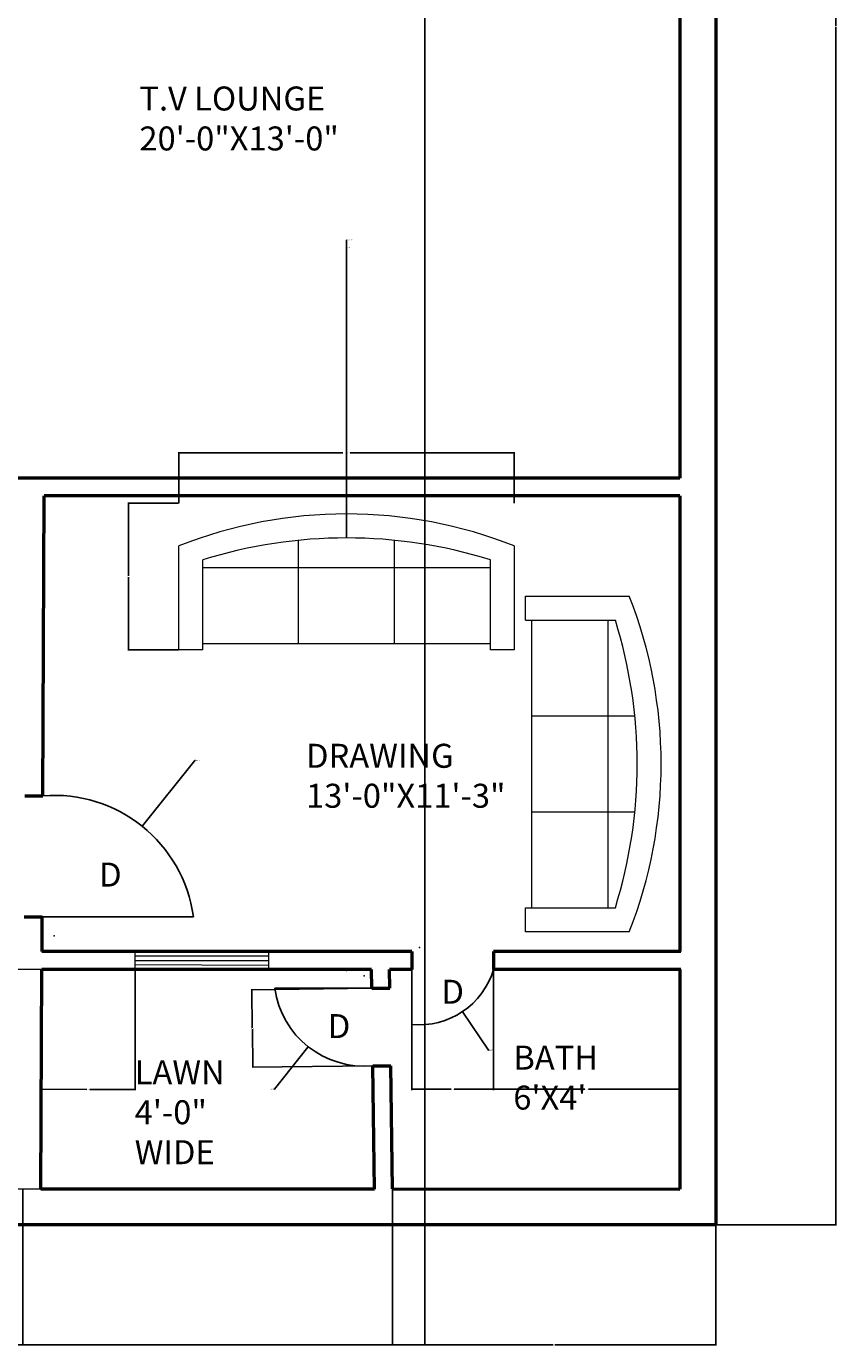
# Model space of a CAD drawing. Units: inches. Extents: x 2341 to 2761, y 2129 to 2789.
# Tile 2 of 4: x 2559 to 2761, y 2129 to 2459. Entities that reach past the tile are written whole.
import ezdxf

# ---------------------------------------------------------------- set-up
doc = ezdxf.new("R2010")
doc.units = ezdxf.units.IN
for name, color, linetype, lineweight in [('A-ANNO-DIMS', 2, 'Continuous', 18), ('A-ANNO-TEXT', 7, 'Continuous', 18), ('A-AREA-IDEN', 7, 'Continuous', 25), ('A-DOOR', 3, 'Continuous', 25), ('A-FURN', 8, 'Continuous', 18), ('A-GLAZ', 4, 'Continuous', 18), ('A-WALL', 7, 'Continuous', 50)]:
    doc.layers.add(name, color=color, linetype=linetype, lineweight=lineweight)
doc.styles.get("Standard").update_dxf_attribs({"font": 'arial.ttf'})
doc.dimstyles.get("Standard").update_dxf_attribs({"dimtxt": 0.18, "dimasz": 0.18, "dimexe": 0.18, "dimexo": 0.0625, "dimgap": 0.09, "dimtad": 0, "dimtih": 1, "dimtoh": 1, "dimdec": 4, "dimzin": 0, "dimdsep": 46, "dimtxsty": 'Standard', "dimcen": 0.09, "dimadec": 0, "dimazin": 0, "dimtfac": 1, "dimtdec": 4, "dimtofl": 0, "dimtmove": 0, "dimatfit": 3, "dimfxl": 1, "dimtolj": 1, "dimtzin": 0, "dimarcsym": 0})

# ---------------------------------------------------------------- blocks, each defined once
blk = doc.blocks.new('Sofa - Roundback 7 ft.')
for p, q in [((-12.00002, -32.4421), (-12.00003, -6.5971)), ((11.99997, -32.4421), (11.99998, -6.5971)), ((-36.000027, -34), (-36.000027, -11.4696)), ((35.99998, -34), (35.99998, -11.4696)), ((-35.999844, -13.3819), (35.9998, -13.3819)), ((-36.000027, -32.4421), (35.99998, -32.4421))]:
    blk.add_line(p, q)
for points in [[(-36.000027, -34), (-42.000027, -34), (-42.000027, -8)], [(41.99998, -8), (41.99998, -34), (35.99998, -34)]]:
    blk.add_lwpolyline(points)
for centre, radius, start, end in [((0, -114.25), 114.25, 68.43141, 111.5686), ((-0.00001, -127.1968), 121.1968, 72.72033, 107.2797)]:
    blk.add_arc(centre, radius, start, end)
blk = doc.blocks.new('WIN-33IN-NARROW')
for p, q in [((0, 3.43), (33.34, 3.43)), ((0, 2.27), (33.34, 2.27)), ((0, 1.23), (33.34, 1.12))]:
    blk.add_line(p, q)
blk.add_lwpolyline([(0, 4.54), (33.34, 4.54), (33.34, 0), (0, 0)], close=True)
blk = doc.blocks.new('*D9')
at = {"layer": 'A-ANNO-DIMS', "color": 0, "lineweight": -2, "transparency": 16777216}
for p, q in [((2596.77, 2339.82), (2596.77, 2352.54)), ((2596.95, 2352.36), (2637.86, 2352.36)), ((2680.59, 2352.36), (2639.67, 2352.36)), ((2680.77, 2339.82), (2680.77, 2352.54))]:
    blk.add_line(p, q, dxfattribs=at)
at = {"layer": 'A-ANNO-DIMS', "color": 0, "transparency": 16777216}
for points in [[(2596.95, 2352.39), (2596.95, 2352.33), (2596.77, 2352.36)], [(2680.59, 2352.39), (2680.59, 2352.33), (2680.77, 2352.36)]]:
    blk.add_solid(points, dxfattribs=at)
at = {"layer": 'Defpoints', "color": 0, "transparency": 16777216}
for p in [(2680.77, 2352.36), (2596.77, 2339.76), (2680.77, 2339.76)]:
    blk.add_point(p, dxfattribs=at)
at = {"layer": 'A-ANNO-DIMS', "color": 0, "transparency": 16777216, "insert": (2638.77, 2352.36), "char_height": 0.18, "attachment_point": 5}
blk.add_mtext('\\A1;SOFA 84 TYP.', dxfattribs=at)
blk = doc.blocks.new('*D10')
at = {"layer": 'A-ANNO-DIMS', "color": 0, "lineweight": -2, "transparency": 16777216}
for p, q in [((2596.71, 2339.76), (2583.99, 2339.76)), ((2584.17, 2339.58), (2584.17, 2321.61)), ((2584.17, 2303.27), (2584.17, 2321.24)), ((2596.71, 2303.09), (2583.99, 2303.09))]:
    blk.add_line(p, q, dxfattribs=at)
at = {"layer": 'A-ANNO-DIMS', "color": 0, "transparency": 16777216}
for points in [[(2584.14, 2339.58), (2584.2, 2339.58), (2584.17, 2339.76)], [(2584.14, 2303.27), (2584.2, 2303.27), (2584.17, 2303.09)]]:
    blk.add_solid(points, dxfattribs=at)
at = {"layer": 'Defpoints', "color": 0, "transparency": 16777216}
for p in [(2584.17, 2339.76), (2596.77, 2339.76), (2596.77, 2303.09)]:
    blk.add_point(p, dxfattribs=at)
at = {"layer": 'A-ANNO-DIMS', "color": 0, "transparency": 16777216, "insert": (2584.17, 2321.42), "char_height": 0.18, "attachment_point": 5}
blk.add_mtext('\\A1;37 TYP.', dxfattribs=at)
blk = doc.blocks.new('*D12')
at = {"layer": 'A-ANNO-DIMS', "color": 0, "lineweight": -2, "transparency": 16777216}
for p, q in [((2731.3, 2759.12), (2761.44, 2759.12)), ((2761.26, 2758.94), (2761.26, 2459.3)), ((2761.26, 2159.3), (2761.26, 2458.94)), ((2731.3, 2159.12), (2761.44, 2159.12))]:
    blk.add_line(p, q, dxfattribs=at)
at = {"layer": 'A-ANNO-DIMS', "color": 0, "transparency": 16777216}
for points in [[(2761.23, 2758.94), (2761.29, 2758.94), (2761.26, 2759.12)], [(2761.23, 2159.3), (2761.29, 2159.3), (2761.26, 2159.12)]]:
    blk.add_solid(points, dxfattribs=at)
at = {"layer": 'Defpoints', "color": 0, "transparency": 16777216}
for p in [(2731.24, 2759.12), (2761.26, 2759.12), (2731.24, 2159.12)]:
    blk.add_point(p, dxfattribs=at)
at = {"layer": 'A-ANNO-DIMS', "color": 0, "transparency": 16777216, "insert": (2761.26, 2459.12), "char_height": 0.18, "attachment_point": 5}
blk.add_mtext('\\A1;600', dxfattribs=at)
blk = doc.blocks.new('*D17')
at = {"layer": 'A-ANNO-DIMS', "color": 0, "lineweight": -2, "transparency": 16777216}
for p, q in [((2444.74, 2750.05), (2444.74, 2128.92)), ((2658.39, 2749.97), (2658.39, 2128.92)), ((2444.92, 2129.1), (2551.1, 2129.1)), ((2658.21, 2129.1), (2552.03, 2129.1))]:
    blk.add_line(p, q, dxfattribs=at)
at = {"layer": 'A-ANNO-DIMS', "color": 0, "transparency": 16777216}
for points in [[(2444.92, 2129.13), (2444.92, 2129.07), (2444.74, 2129.1)], [(2658.21, 2129.13), (2658.21, 2129.07), (2658.39, 2129.1)]]:
    blk.add_solid(points, dxfattribs=at)
at = {"layer": 'Defpoints', "color": 0, "transparency": 16777216}
for p in [(2444.74, 2750.12), (2658.39, 2750.04), (2658.39, 2129.1)]:
    blk.add_point(p, dxfattribs=at)
at = {"layer": 'A-ANNO-DIMS', "color": 0, "transparency": 16777216, "insert": (2551.56, 2129.1), "char_height": 0.18, "attachment_point": 5}
blk.add_mtext('\\A1;213.65', dxfattribs=at)
blk = doc.blocks.new('*D25')
at = {"layer": 'A-ANNO-DIMS', "color": 0, "lineweight": -2, "transparency": 16777216}
for p, q in [((2557.74, 2168.07), (2557.74, 2128.92)), ((2650.24, 2168.1), (2650.24, 2128.92)), ((2557.92, 2129.1), (2603.67, 2129.1)), ((2650.06, 2129.1), (2604.32, 2129.1))]:
    blk.add_line(p, q, dxfattribs=at)
at = {"layer": 'A-ANNO-DIMS', "color": 0, "transparency": 16777216}
for points in [[(2557.92, 2129.13), (2557.92, 2129.07), (2557.74, 2129.1)], [(2650.06, 2129.13), (2650.06, 2129.07), (2650.24, 2129.1)]]:
    blk.add_solid(points, dxfattribs=at)
at = {"layer": 'Defpoints', "color": 0, "transparency": 16777216}
for p in [(2557.74, 2168.13), (2650.24, 2168.16), (2650.24, 2129.1)]:
    blk.add_point(p, dxfattribs=at)
at = {"layer": 'A-ANNO-DIMS', "color": 0, "transparency": 16777216, "insert": (2603.99, 2129.1), "char_height": 0.18, "attachment_point": 5}
blk.add_mtext('\\A1;92.5', dxfattribs=at)
blk = doc.blocks.new('*D26')
at = {"layer": 'A-ANNO-DIMS', "color": 0, "lineweight": -2, "transparency": 16777216}
for p, q in [((2650.24, 2168.1), (2650.24, 2128.92)), ((2731.24, 2159.06), (2731.24, 2128.92)), ((2650.42, 2129.1), (2690.54, 2129.1)), ((2731.06, 2129.1), (2690.94, 2129.1))]:
    blk.add_line(p, q, dxfattribs=at)
at = {"layer": 'A-ANNO-DIMS', "color": 0, "transparency": 16777216}
for points in [[(2650.42, 2129.13), (2650.42, 2129.07), (2650.24, 2129.1)], [(2731.06, 2129.13), (2731.06, 2129.07), (2731.24, 2129.1)]]:
    blk.add_solid(points, dxfattribs=at)
at = {"layer": 'Defpoints', "color": 0, "transparency": 16777216}
for p in [(2650.24, 2168.16), (2731.24, 2159.12), (2731.24, 2129.1)]:
    blk.add_point(p, dxfattribs=at)
at = {"layer": 'A-ANNO-DIMS', "color": 0, "transparency": 16777216, "insert": (2690.74, 2129.1), "char_height": 0.18, "attachment_point": 5}
blk.add_mtext('\\A1;81', dxfattribs=at)
blk = doc.blocks.new('*D30')
at = {"layer": 'A-ANNO-DIMS', "color": 0, "lineweight": -2, "transparency": 16777216}
for p, q in [((2562.45, 2223.1), (2532.31, 2223.25)), ((2532.49, 2223.06), (2532.36, 2195.94)), ((2532.22, 2168.45), (2532.36, 2195.58)), ((2562.18, 2168.12), (2532.04, 2168.27))]:
    blk.add_line(p, q, dxfattribs=at)
at = {"layer": 'A-ANNO-DIMS', "color": 0, "transparency": 16777216}
for points in [[(2532.46, 2223.06), (2532.52, 2223.06), (2532.49, 2223.24)], [(2532.19, 2168.45), (2532.25, 2168.45), (2532.22, 2168.27)]]:
    blk.add_solid(points, dxfattribs=at)
at = {"layer": 'Defpoints', "color": 0, "transparency": 16777216}
for p in [(2532.49, 2223.24), (2562.51, 2223.1), (2562.24, 2168.12)]:
    blk.add_point(p, dxfattribs=at)
at = {"layer": 'A-ANNO-DIMS', "color": 0, "transparency": 16777216, "insert": (2532.36, 2195.76), "char_height": 0.18, "attachment_point": 5}
blk.add_mtext('\\A1;54.97', dxfattribs=at)
blk = doc.blocks.new('*D35')
at = {"layer": 'A-ANNO-DIMS', "color": 0, "lineweight": -2, "transparency": 16777216}
for p, q in [((2562.51, 2223.03), (2562.46, 2192.9)), ((2585.87, 2222.99), (2585.82, 2192.85)), ((2562.64, 2193.08), (2573.75, 2193.06)), ((2585.64, 2193.04), (2574.54, 2193.05))]:
    blk.add_line(p, q, dxfattribs=at)
at = {"layer": 'A-ANNO-DIMS', "color": 0, "transparency": 16777216}
for points in [[(2562.64, 2193.11), (2562.64, 2193.05), (2562.46, 2193.08)], [(2585.64, 2193.07), (2585.64, 2193.01), (2585.82, 2193.03)]]:
    blk.add_solid(points, dxfattribs=at)
at = {"layer": 'Defpoints', "color": 0, "transparency": 16777216}
for p in [(2562.51, 2223.1), (2585.87, 2223.05), (2562.46, 2193.08)]:
    blk.add_point(p, dxfattribs=at)
at = {"layer": 'A-ANNO-DIMS', "color": 0, "transparency": 16777216, "insert": (2574.14, 2193.06), "char_height": 0.18, "attachment_point": 5}
blk.add_mtext('\\A1;23.36', dxfattribs=at)
blk = doc.blocks.new('*D53')
at = {"layer": 'A-ANNO-DIMS', "color": 0, "lineweight": -2, "transparency": 16777216}
for p, q in [((2655.1, 2223.03), (2655.1, 2192.9)), ((2675.59, 2223.03), (2675.59, 2192.9)), ((2655.28, 2193.08), (2664.95, 2193.08)), ((2675.41, 2193.08), (2665.74, 2193.08))]:
    blk.add_line(p, q, dxfattribs=at)
at = {"layer": 'A-ANNO-DIMS', "color": 0, "transparency": 16777216}
for points in [[(2655.28, 2193.11), (2655.28, 2193.05), (2655.1, 2193.08)], [(2675.41, 2193.11), (2675.41, 2193.05), (2675.59, 2193.08)]]:
    blk.add_solid(points, dxfattribs=at)
at = {"layer": 'Defpoints', "color": 0, "transparency": 16777216}
for p in [(2655.1, 2223.1), (2675.59, 2223.1), (2655.1, 2193.08)]:
    blk.add_point(p, dxfattribs=at)
at = {"layer": 'A-ANNO-DIMS', "color": 0, "transparency": 16777216, "insert": (2665.34, 2193.08), "char_height": 0.18, "attachment_point": 5}
blk.add_mtext('\\A1;20.49', dxfattribs=at)
blk = doc.blocks.new('*D54')
at = {"layer": 'A-ANNO-DIMS', "color": 0, "lineweight": -2, "transparency": 16777216}
for p, q in [((2675.59, 2223.03), (2675.59, 2192.9)), ((2722.24, 2223.03), (2722.24, 2192.9)), ((2675.77, 2193.08), (2698.45, 2193.08)), ((2722.06, 2193.08), (2699.38, 2193.08))]:
    blk.add_line(p, q, dxfattribs=at)
at = {"layer": 'A-ANNO-DIMS', "color": 0, "transparency": 16777216}
for points in [[(2675.77, 2193.11), (2675.77, 2193.05), (2675.59, 2193.08)], [(2722.06, 2193.11), (2722.06, 2193.05), (2722.24, 2193.08)]]:
    blk.add_solid(points, dxfattribs=at)
at = {"layer": 'Defpoints', "color": 0, "transparency": 16777216}
for p in [(2675.59, 2223.1), (2722.24, 2223.1), (2675.59, 2193.08)]:
    blk.add_point(p, dxfattribs=at)
at = {"layer": 'A-ANNO-DIMS', "color": 0, "transparency": 16777216, "insert": (2698.91, 2193.08), "char_height": 0.18, "attachment_point": 5}
blk.add_mtext('\\A1;46.655', dxfattribs=at)
blk = doc.blocks.new('*D55')
at = {"layer": 'A-ANNO-DIMS', "color": 0, "lineweight": -2, "transparency": 16777216}
for p, q in [((2645.01, 2218.37), (2614.88, 2217.97)), ((2615.06, 2217.79), (2615.18, 2208.46)), ((2615.31, 2198.77), (2615.19, 2208.1)), ((2645.27, 2198.99), (2615.13, 2198.59))]:
    blk.add_line(p, q, dxfattribs=at)
at = {"layer": 'A-ANNO-DIMS', "color": 0, "transparency": 16777216}
for points in [[(2615.09, 2217.79), (2615.03, 2217.79), (2615.06, 2217.97)], [(2615.34, 2198.77), (2615.28, 2198.77), (2615.31, 2198.59)]]:
    blk.add_solid(points, dxfattribs=at)
at = {"layer": 'Defpoints', "color": 0, "transparency": 16777216}
for p in [(2615.06, 2217.97), (2645.07, 2218.37), (2645.33, 2198.99)]:
    blk.add_point(p, dxfattribs=at)
at = {"layer": 'A-ANNO-DIMS', "color": 0, "transparency": 16777216, "insert": (2615.19, 2208.28), "char_height": 0.18, "attachment_point": 5}
blk.add_mtext('\\A1;19.386', dxfattribs=at)
blk = doc.blocks.new('*D60')
at = {"layer": 'A-ANNO-DIMS', "color": 0, "lineweight": -2, "transparency": 16777216}
for p, q in [((2638.95, 2403.81), (2638.77, 2403.81)), ((2638.77, 2403.81), (2638.77, 2331.27)), ((2638.68, 2209.89), (2638.86, 2209.89)), ((2638.77, 2209.8), (2638.77, 2209.98))]:
    blk.add_line(p, q, dxfattribs=at)
at = {"layer": 'A-ANNO-DIMS', "color": 0, "transparency": 16777216}
blk.add_solid([(2638.74, 2331.27), (2638.8, 2331.27), (2638.77, 2331.09)], dxfattribs=at)
at = {"layer": 'Defpoints', "color": 0, "transparency": 16777216}
for p in [(2638.77, 2331.09), (2638.77, 2209.89)]:
    blk.add_point(p, dxfattribs=at)
at = {"layer": 'A-ANNO-DIMS', "color": 0, "transparency": 16777216, "insert": (2639.62, 2403.81), "char_height": 0.18, "attachment_point": 5}
blk.add_mtext('\\A1;2X R121.2', dxfattribs=at)
blk = doc.blocks.new('*D61')
at = {"layer": 'A-ANNO-DIMS', "color": 0, "lineweight": -2, "transparency": 16777216}
for p, q in [((2638.95, 2405.64), (2638.77, 2405.64)), ((2638.77, 2405.64), (2638.77, 2337.27)), ((2638.68, 2222.84), (2638.86, 2222.84)), ((2638.77, 2222.75), (2638.77, 2222.93))]:
    blk.add_line(p, q, dxfattribs=at)
at = {"layer": 'A-ANNO-DIMS', "color": 0, "transparency": 16777216}
blk.add_solid([(2638.74, 2337.27), (2638.8, 2337.27), (2638.77, 2337.09)], dxfattribs=at)
at = {"layer": 'Defpoints', "color": 0, "transparency": 16777216}
for p in [(2638.77, 2337.09), (2638.77, 2222.84)]:
    blk.add_point(p, dxfattribs=at)
at = {"layer": 'A-ANNO-DIMS', "color": 0, "transparency": 16777216, "insert": (2639.7, 2405.64), "char_height": 0.18, "attachment_point": 5}
blk.add_mtext('\\A1;2X R114.25', dxfattribs=at)
blk = doc.blocks.new('*D68')
at = {"layer": 'A-ANNO-DIMS', "color": 0, "lineweight": -2, "transparency": 16777216}
for p, q in [((2600.8, 2275.37), (2587.71, 2259.06)), ((2600.98, 2275.37), (2600.8, 2275.37)), ((2565.51, 2231.51), (2565.69, 2231.51)), ((2565.6, 2231.42), (2565.6, 2231.6))]:
    blk.add_line(p, q, dxfattribs=at)
at = {"layer": 'A-ANNO-DIMS', "color": 0, "transparency": 16777216}
blk.add_solid([(2587.69, 2259.08), (2587.73, 2259.04), (2587.6, 2258.92)], dxfattribs=at)
at = {"layer": 'Defpoints', "color": 0, "transparency": 16777216}
for p in [(2587.6, 2258.92), (2565.6, 2231.51)]:
    blk.add_point(p, dxfattribs=at)
at = {"layer": 'A-ANNO-DIMS', "color": 0, "transparency": 16777216, "insert": (2601.53, 2275.37), "char_height": 0.18, "attachment_point": 5}
blk.add_mtext('\\A1;R35.145', dxfattribs=at)
blk = doc.blocks.new('*D72')
at = {"layer": 'A-ANNO-DIMS', "color": 0, "lineweight": -2, "transparency": 16777216}
for p, q in [((2643.07, 2221.47), (2643.25, 2221.47)), ((2643.16, 2221.38), (2643.16, 2221.56)), ((2620.76, 2193.11), (2629.05, 2203.6)), ((2620.58, 2193.11), (2620.76, 2193.11))]:
    blk.add_line(p, q, dxfattribs=at)
at = {"layer": 'A-ANNO-DIMS', "color": 0, "transparency": 16777216}
blk.add_solid([(2629.03, 2203.62), (2629.07, 2203.58), (2629.16, 2203.74)], dxfattribs=at)
at = {"layer": 'Defpoints', "color": 0, "transparency": 16777216}
for p in [(2643.16, 2221.47), (2629.16, 2203.74)]:
    blk.add_point(p, dxfattribs=at)
at = {"layer": 'A-ANNO-DIMS', "color": 0, "transparency": 16777216, "insert": (2620.1, 2193.11), "char_height": 0.18, "attachment_point": 5}
blk.add_mtext('\\A1;R22.59', dxfattribs=at)
blk = doc.blocks.new('*D73')
at = {"layer": 'A-ANNO-DIMS', "color": 0, "lineweight": -2, "transparency": 16777216}
for p, q in [((2656.92, 2228.61), (2657.1, 2228.61)), ((2657.01, 2228.52), (2657.01, 2228.7)), ((2674.3, 2202.88), (2667.92, 2212.38)), ((2674.48, 2202.88), (2674.3, 2202.88))]:
    blk.add_line(p, q, dxfattribs=at)
at = {"layer": 'A-ANNO-DIMS', "color": 0, "transparency": 16777216}
blk.add_solid([(2667.94, 2212.4), (2667.89, 2212.36), (2667.82, 2212.53)], dxfattribs=at)
at = {"layer": 'Defpoints', "color": 0, "transparency": 16777216}
for p in [(2657.01, 2228.61), (2667.82, 2212.53)]:
    blk.add_point(p, dxfattribs=at)
at = {"layer": 'A-ANNO-DIMS', "color": 0, "transparency": 16777216, "insert": (2675.03, 2202.88), "char_height": 0.18, "attachment_point": 5}
blk.add_mtext('\\A1;R19.375', dxfattribs=at)

msp = doc.modelspace()

# ---------------------------------------------------------------- linework, layer by layer
at = {"layer": 'A-DOOR'}
for p, q in [((2562.5798, 2236.2899), (2600.4188, 2236.2899)), ((2655.0973, 2223.096), (2655.0973, 2209.3312)), ((2645.0739, 2218.3709), (2620.787, 2218.3709))]:
    msp.add_line(p, q, dxfattribs=at)
for centre, radius, start, end in [((2565.6002, 2231.5125), 35.1449, 7.812565, 94.684937), ((2657.0121, 2228.6113), 19.3749, 264.328177, 343.461296), ((2643.1616, 2221.4705), 22.5883, 187.887216, 275.51305)]:
    msp.add_arc(centre, radius, start, end, dxfattribs=at)
at = {"layer": 'A-WALL'}
for p, q in [((2731.242, 2759.1219), (2731.242, 2159.1219)), ((2722.2419, 2497.5958), (2722.2379, 2346.0958)), ((2722.2379, 2346.0958), (2532.3567, 2346.0958)), ((2558.6238, 2346.0958), (2558.6239, 2346.1181)), ((2562.7297, 2266.54), (2563.1015, 2341.5958)), ((2722.2379, 2341.5958), (2563.1015, 2341.5958)), ((2722.2379, 2341.5958), (2722.2406, 2227.596)), ((2558.2296, 2266.54), (2562.7297, 2266.54)), ((2558.0798, 2236.2899), (2562.5798, 2236.2899)), ((2562.5368, 2227.596), (2562.5798, 2236.2899)), ((2655.0973, 2227.596), (2562.5145, 2227.596)), ((2655.0973, 2227.596), (2655.0973, 2223.096)), ((2722.464, 2227.596), (2675.5855, 2227.596)), ((2675.5855, 2227.596), (2675.5855, 2223.096)), ((2562.242, 2168.1065), (2562.5145, 2223.096)), ((2645.0119, 2223.0362), (2562.5145, 2223.096)), ((2645.0739, 2218.3709), (2645.0119, 2223.0362)), ((2649.5743, 2218.3709), (2649.5115, 2223.096)), ((2655.0973, 2223.096), (2649.5115, 2223.096)), ((2722.464, 2223.096), (2675.5855, 2223.096)), ((2722.2407, 2223.096), (2722.242, 2168.1219)), ((2645.0739, 2218.3709), (2649.5743, 2218.3709)), ((2645.7425, 2168.1007), (2645.3317, 2198.9867)), ((2645.3317, 2198.9867), (2649.8321, 2198.9867)), ((2650.2421, 2168.1606), (2649.8321, 2198.9867)), ((2645.7422, 2168.1219), (2562.2421, 2168.1219)), ((2650.2421, 2168.1606), (2722.242, 2168.1219)), ((2731.242, 2159.1219), (2537.006, 2159.1219))]:
    msp.add_line(p, q, dxfattribs=at)

# ---------------------------------------------------------------- block references
at = {"layer": 'A-FURN'}
msp.add_blockref('Sofa - Roundback 7 ft.', (2638.7698, 2337.0912), dxfattribs=at)
at = {"layer": 'A-FURN', "rotation": 270}
msp.add_blockref('Sofa - Roundback 7 ft.', (2717.5357, 2274.5241), dxfattribs=at)
at = {"layer": 'A-GLAZ'}
msp.add_blockref('WIN-33IN-NARROW', (2585.873, 2223.055), dxfattribs=at)

# ---------------------------------------------------------------- texts
at = {"layer": 'A-ANNO-TEXT', "char_height": 6, "attachment_point": 1}
for insert in [(2576.8331, 2249.8152), (2662.5323, 2220.5011), (2634.0759, 2211.9016)]:
    msp.add_mtext_dynamic_manual_height_columns('D', width=9.002909, gutter_width=12.5, heights=[0], dxfattribs=dict(at, insert=insert))
at = {"layer": 'A-AREA-IDEN', "char_height": 6, "attachment_point": 1}
for s, width, insert in [('T.V LOUNGE\\P20\'-0"X13\'-0"', 96.613534, (2586.9046, 2444.0888)), ('DRAWING \\P13\'-0"X11\'-3"', 59.833005, (2628.6328, 2279.56)), ("BATH \\P6'X4'", 44.392283, (2680.5248, 2204.0067)), ('LAWN 4\'-0" WIDE', 28.56042, (2585.7319, 2200.3444))]:
    msp.add_mtext_dynamic_manual_height_columns(s, width=width, gutter_width=12.5, heights=[0], dxfattribs=dict(at, insert=insert))

# ---------------------------------------------------------------- dimensions: what is measured, and where the dimension line sits
at = {"layer": 'A-ANNO-DIMS'}
for base, p1, p2, angle, override, picture, middle in [((2761.262, 2759.1219), (2731.242, 2159.1219), (2731.242, 2759.1219), 90, {"dimdec": 0, "dimlfac": 1, "dimrnd": 0, "dimzin": 0, "dimdsep": 46, "dimlunit": 2}, '*D12', (2761.262, 2459.1219)), ((2532.4948, 2223.2447), (2562.2421, 2168.1219), (2562.5145, 2223.096), 89.716153, {"dimdec": 2, "dimlfac": 1, "dimrnd": 0, "dimzin": 0, "dimdsep": 46, "dimlunit": 2}, '*D30', (2532.3587, 2195.7577)), ((2562.4616, 2193.076), (2585.8726, 2223.0549), (2562.5145, 2223.096), 179.899111, {"dimdec": 2, "dimlfac": 1, "dimrnd": 0, "dimzin": 0, "dimdsep": 46, "dimlunit": 2}, '*D35', (2574.1407, 2193.0555)), ((2655.0973, 2193.076), (2675.5855, 2223.096), (2655.0973, 2223.096), 180, {"dimdec": 2, "dimlfac": 1, "dimrnd": 0, "dimzin": 0, "dimdsep": 46, "dimlunit": 2}, '*D53', (2665.3414, 2193.076)), ((2675.5855, 2193.076), (2722.2407, 2223.096), (2675.5855, 2223.096), 180, {"dimdec": 3, "dimlfac": 1, "dimrnd": 0, "dimzin": 0, "dimdsep": 46, "dimlunit": 2}, '*D54', (2698.9131, 2193.076)), ((2615.0566, 2217.9717), (2645.3317, 2198.9867), (2645.0739, 2218.3709), 90.761924, {"dimdec": 3, "dimlfac": 1, "dimrnd": 0, "dimzin": 0, "dimdsep": 46, "dimlunit": 2}, '*D55', (2615.1855, 2208.2796))]:
    dim = msp.add_linear_dim(base=base, p1=p1, p2=p2, angle=angle, dimstyle='Standard', override=override, dxfattribs=at)
    dim.commit()
    dim.dimension.update_dxf_attribs({"geometry": picture, "text_midpoint": middle})
for base, p1, p2, override, picture, middle in [((2658.3873, 2129.1019), (2444.742, 2750.1173), (2658.3873, 2750.0366), {"dimdec": 2, "dimlfac": 1, "dimrnd": 0, "dimzin": 0, "dimdsep": 46, "dimlunit": 2}, '*D17', (2551.5646, 2129.1019)), ((2650.2421, 2129.1019), (2557.7421, 2168.1288), (2650.2421, 2168.1606), {"dimdec": 1, "dimlfac": 1, "dimrnd": 0, "dimzin": 0, "dimdsep": 46, "dimlunit": 2}, '*D25', (2603.9921, 2129.1019)), ((2731.242, 2129.1019), (2650.2421, 2168.1606), (2731.242, 2159.1219), {"dimdec": 0, "dimlfac": 1, "dimrnd": 0, "dimzin": 0, "dimdsep": 46, "dimlunit": 2}, '*D26', (2690.742, 2129.1019))]:
    dim = msp.add_linear_dim(base=base, p1=p1, p2=p2, dimstyle='Standard', override=override, dxfattribs=at)
    dim.commit()
    dim.dimension.update_dxf_attribs({"geometry": picture, "text_midpoint": middle})
for center, mpoint, override, picture, middle in [((2638.7698, 2222.8412), (2638.77, 2337.0912), {"dimdec": 2, "dimlfac": 1, "dimrnd": 0, "dimzin": 0, "dimdsep": 46, "dimlunit": 2}, '*D61', (2639.6955, 2405.6412)), ((2638.7698, 2209.8944), (2638.77, 2331.0912), {"dimdec": 1, "dimlfac": 1, "dimrnd": 0, "dimzin": 0, "dimdsep": 46, "dimlunit": 2}, '*D60', (2639.624, 2403.8092))]:
    dim = msp.add_radius_dim(center=center, mpoint=mpoint, text='2X <>', dimstyle='Standard', override=override, dxfattribs=at)
    dim.commit()
    dim.dimension.update_dxf_attribs({"geometry": picture, "text_midpoint": middle, "dimtype": 164})
dim = msp.add_linear_dim(base=(2680.7698, 2352.3578), p1=(2596.7697, 2339.7578), p2=(2680.7698, 2339.7578), text='SOFA <> TYP.', dimstyle='Standard', override={"dimdec": 0, "dimlfac": 1, "dimrnd": 0, "dimzin": 0, "dimdsep": 46, "dimlunit": 2}, dxfattribs=at)
dim.commit()
dim.dimension.update_dxf_attribs({"geometry": '*D9', "text_midpoint": (2638.7697, 2352.3578)})
dim = msp.add_linear_dim(base=(2584.1697, 2339.7578), p1=(2596.7697, 2303.0912), p2=(2596.7697, 2339.7578), angle=90, text='<> TYP.', dimstyle='Standard', override={"dimdec": 0, "dimlfac": 1, "dimrnd": 0, "dimzin": 0, "dimdsep": 46, "dimlunit": 2}, dxfattribs=at)
dim.commit()
dim.dimension.update_dxf_attribs({"geometry": '*D10', "text_midpoint": (2584.1697, 2321.4245)})
for center, mpoint, override, picture, middle in [((2565.6002, 2231.5125), (2587.5989, 2258.9209), {"dimdec": 3, "dimlfac": 1, "dimrnd": 0, "dimzin": 0, "dimdsep": 46, "dimlunit": 2}, '*D68', (2601.5286, 2275.3659)), ((2657.0121, 2228.6113), (2667.817, 2212.529), {"dimdec": 3, "dimlfac": 1, "dimrnd": 0, "dimzin": 0, "dimdsep": 46, "dimlunit": 2}, '*D73', (2675.0304, 2202.8796)), ((2643.1616, 2221.4705), (2629.1618, 2203.7438), {"dimdec": 2, "dimlfac": 1, "dimrnd": 0, "dimzin": 0, "dimdsep": 46, "dimlunit": 2}, '*D72', (2620.1019, 2193.1077))]:
    dim = msp.add_radius_dim(center=center, mpoint=mpoint, dimstyle='Standard', override=override, dxfattribs=at)
    dim.commit()
    dim.dimension.update_dxf_attribs({"geometry": picture, "text_midpoint": middle, "dimtype": 164})

doc.saveas('drawing.dxf')
